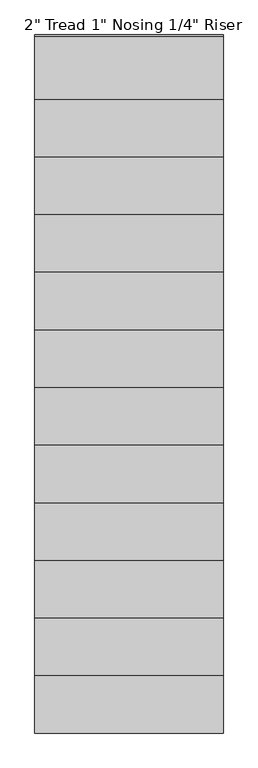
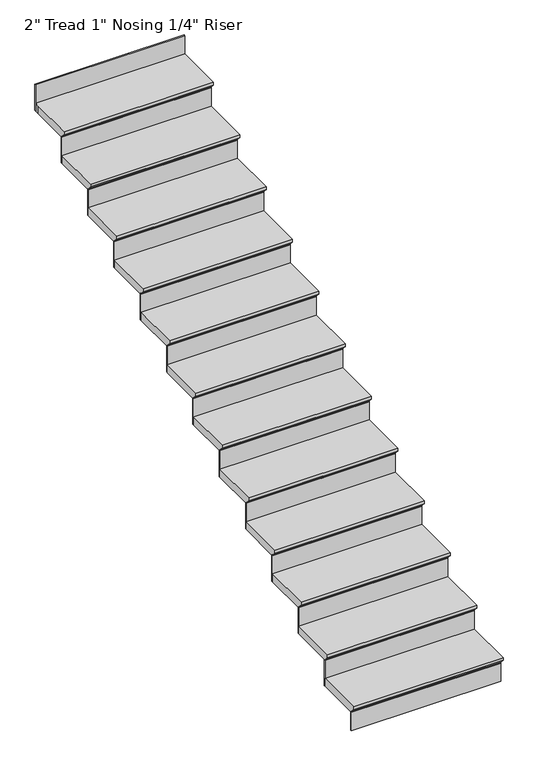
"""IFC4 building model written with IfcOpenShell, lengths in millimetres: stair flight geometry."""

from ifc_helpers import new_model, si_unit, origin, place, context, project, spatial, faceted_brep, source, transform, mapped, element, save


def stair_flight_f72f160c(model_context):
    return source(origin(), model_context, "Body", "Brep", [
        faceted_brep([(-2703.0415084, 19841.9216096, 43672.9005799), (-2703.0415084, 19841.9216096, 43691.9505799), (-3617.4415084, 19841.9216096, 43691.9505799), (-3617.4415084, 19841.9216096, 43672.9005799), (-2703.0415084, 19867.3216096, 43647.5005799), (-3617.4415084, 19867.3216096, 43647.5005799), (-2703.0415084, 20146.7216096, 43691.9505799), (-3617.4415084, 20146.7216096, 43691.9505799), (-3617.4415084, 19867.3216096, 43641.1505799), (-3617.4415084, 20146.7216096, 43641.1505799), (-2703.0415084, 20146.7216096, 43641.1505799), (-2703.0415084, 19867.3216096, 43641.1505799)], [[[0, 1, 2, 3]], [[4, 0, 3, 5]], [[2, 1, 6, 7]], [[8, 9, 10, 11]], [[2, 7, 9, 8, 5, 3]], [[8, 11, 4, 5]], [[6, 1, 0, 4, 11, 10]], [[7, 6, 10, 9]]]),
        faceted_brep([(-2703.0415084, 19867.3216096, 43641.1505799), (-2703.0415084, 19867.3216096, 43522.6172466), (-2703.0415084, 19873.6716096, 43522.6172466), (-2703.0415084, 19873.6716096, 43641.1505799), (-3617.4415084, 19867.3216096, 43641.1505799), (-3617.4415084, 19873.6716096, 43641.1505799), (-3617.4415084, 19873.6716096, 43522.6172466), (-3617.4415084, 19867.3216096, 43522.6172466)], [[[0, 1, 2, 3]], [[4, 5, 6, 7]], [[1, 0, 4, 7]], [[2, 1, 7, 6]], [[3, 2, 6, 5]], [[0, 3, 5, 4]]]),
        faceted_brep([(-2703.0415084, 20146.7216096, 43810.4839133), (-2703.0415084, 20146.7216096, 43641.1505799), (-2703.0415084, 20153.0716096, 43641.1505799), (-2703.0415084, 20153.0716096, 43810.4839133), (-3617.4415084, 20146.7216096, 43810.4839133), (-3617.4415084, 20153.0716096, 43810.4839133), (-3617.4415084, 20153.0716096, 43641.1505799), (-3617.4415084, 20146.7216096, 43641.1505799)], [[[0, 1, 2, 3]], [[4, 5, 6, 7]], [[1, 0, 4, 7]], [[2, 1, 7, 6]], [[3, 2, 6, 5]], [[0, 3, 5, 4]]]),
        faceted_brep([(-3617.4415084, 20121.3216096, 43861.2839133), (-2703.0415084, 20121.3216096, 43861.2839133), (-2703.0415084, 20426.1216096, 43861.2839133), (-3617.4415084, 20426.1216096, 43861.2839133), (-3617.4415084, 20146.7216096, 43810.4839133), (-3617.4415084, 20426.1216096, 43810.4839133), (-2703.0415084, 20426.1216096, 43810.4839133), (-2703.0415084, 20146.7216096, 43810.4839133), (-3617.4415084, 20146.7216096, 43816.8339133), (-3617.4415084, 20121.3216096, 43842.2339133), (-2703.0415084, 20146.7216096, 43816.8339133), (-2703.0415084, 20121.3216096, 43842.2339133)], [[[0, 1, 2, 3]], [[4, 5, 6, 7]], [[0, 3, 5, 4, 8, 9]], [[4, 7, 10, 8]], [[2, 1, 11, 10, 7, 6]], [[3, 2, 6, 5]], [[11, 1, 0, 9]], [[10, 11, 9, 8]]]),
        faceted_brep([(-2703.0415084, 20426.1216096, 43979.8172466), (-2703.0415084, 20426.1216096, 43810.4839133), (-2703.0415084, 20432.4716096, 43810.4839133), (-2703.0415084, 20432.4716096, 43979.8172466), (-3617.4415084, 20426.1216096, 43979.8172466), (-3617.4415084, 20432.4716096, 43979.8172466), (-3617.4415084, 20432.4716096, 43810.4839133), (-3617.4415084, 20426.1216096, 43810.4839133)], [[[0, 1, 2, 3]], [[4, 5, 6, 7]], [[1, 0, 4, 7]], [[2, 1, 7, 6]], [[3, 2, 6, 5]], [[0, 3, 5, 4]]]),
        faceted_brep([(-3617.4415084, 20400.7216096, 44030.6172466), (-2703.0415084, 20400.7216096, 44030.6172466), (-2703.0415084, 20705.5216096, 44030.6172466), (-3617.4415084, 20705.5216096, 44030.6172466), (-3617.4415084, 20426.1216096, 43979.8172466), (-3617.4415084, 20705.5216096, 43979.8172466), (-2703.0415084, 20705.5216096, 43979.8172466), (-2703.0415084, 20426.1216096, 43979.8172466), (-3617.4415084, 20426.1216096, 43986.1672466), (-3617.4415084, 20400.7216096, 44011.5672466), (-2703.0415084, 20426.1216096, 43986.1672466), (-2703.0415084, 20400.7216096, 44011.5672466)], [[[0, 1, 2, 3]], [[4, 5, 6, 7]], [[0, 3, 5, 4, 8, 9]], [[4, 7, 10, 8]], [[2, 1, 11, 10, 7, 6]], [[3, 2, 6, 5]], [[11, 1, 0, 9]], [[10, 11, 9, 8]]]),
        faceted_brep([(-2703.0415084, 20705.5216096, 44149.1505799), (-2703.0415084, 20705.5216096, 43979.8172466), (-2703.0415084, 20711.8716096, 43979.8172466), (-2703.0415084, 20711.8716096, 44149.1505799), (-3617.4415084, 20705.5216096, 44149.1505799), (-3617.4415084, 20711.8716096, 44149.1505799), (-3617.4415084, 20711.8716096, 43979.8172466), (-3617.4415084, 20705.5216096, 43979.8172466)], [[[0, 1, 2, 3]], [[4, 5, 6, 7]], [[1, 0, 4, 7]], [[2, 1, 7, 6]], [[3, 2, 6, 5]], [[0, 3, 5, 4]]]),
        faceted_brep([(-3617.4415084, 20680.1216096, 44199.9505799), (-2703.0415084, 20680.1216096, 44199.9505799), (-2703.0415084, 20984.9216096, 44199.9505799), (-3617.4415084, 20984.9216096, 44199.9505799), (-3617.4415084, 20705.5216096, 44149.1505799), (-3617.4415084, 20984.9216096, 44149.1505799), (-2703.0415084, 20984.9216096, 44149.1505799), (-2703.0415084, 20705.5216096, 44149.1505799), (-3617.4415084, 20705.5216096, 44155.5005799), (-3617.4415084, 20680.1216096, 44180.9005799), (-2703.0415084, 20705.5216096, 44155.5005799), (-2703.0415084, 20680.1216096, 44180.9005799)], [[[0, 1, 2, 3]], [[4, 5, 6, 7]], [[0, 3, 5, 4, 8, 9]], [[4, 7, 10, 8]], [[2, 1, 11, 10, 7, 6]], [[3, 2, 6, 5]], [[11, 1, 0, 9]], [[10, 11, 9, 8]]]),
        faceted_brep([(-2703.0415084, 20984.9216096, 44318.4839133), (-2703.0415084, 20984.9216096, 44149.1505799), (-2703.0415084, 20991.2716096, 44149.1505799), (-2703.0415084, 20991.2716096, 44318.4839133), (-3617.4415084, 20984.9216096, 44318.4839133), (-3617.4415084, 20991.2716096, 44318.4839133), (-3617.4415084, 20991.2716096, 44149.1505799), (-3617.4415084, 20984.9216096, 44149.1505799)], [[[0, 1, 2, 3]], [[4, 5, 6, 7]], [[1, 0, 4, 7]], [[2, 1, 7, 6]], [[3, 2, 6, 5]], [[0, 3, 5, 4]]]),
        faceted_brep([(-3617.4415084, 20959.5216096, 44369.2839133), (-2703.0415084, 20959.5216096, 44369.2839133), (-2703.0415084, 21264.3216096, 44369.2839133), (-3617.4415084, 21264.3216096, 44369.2839133), (-3617.4415084, 20984.9216096, 44318.4839133), (-3617.4415084, 21264.3216096, 44318.4839133), (-2703.0415084, 21264.3216096, 44318.4839133), (-2703.0415084, 20984.9216096, 44318.4839133), (-3617.4415084, 20984.9216096, 44324.8339133), (-3617.4415084, 20959.5216096, 44350.2339133), (-2703.0415084, 20984.9216096, 44324.8339133), (-2703.0415084, 20959.5216096, 44350.2339133)], [[[0, 1, 2, 3]], [[4, 5, 6, 7]], [[0, 3, 5, 4, 8, 9]], [[4, 7, 10, 8]], [[2, 1, 11, 10, 7, 6]], [[3, 2, 6, 5]], [[11, 1, 0, 9]], [[10, 11, 9, 8]]]),
        faceted_brep([(-2703.0415084, 21264.3216096, 44487.8172466), (-2703.0415084, 21264.3216096, 44318.4839133), (-2703.0415084, 21270.6716096, 44318.4839133), (-2703.0415084, 21270.6716096, 44487.8172466), (-3617.4415084, 21264.3216096, 44487.8172466), (-3617.4415084, 21270.6716096, 44487.8172466), (-3617.4415084, 21270.6716096, 44318.4839133), (-3617.4415084, 21264.3216096, 44318.4839133)], [[[0, 1, 2, 3]], [[4, 5, 6, 7]], [[1, 0, 4, 7]], [[2, 1, 7, 6]], [[3, 2, 6, 5]], [[0, 3, 5, 4]]]),
        faceted_brep([(-3617.4415084, 21238.9216096, 44538.6172466), (-2703.0415084, 21238.9216096, 44538.6172466), (-2703.0415084, 21543.7216096, 44538.6172466), (-3617.4415084, 21543.7216096, 44538.6172466), (-3617.4415084, 21264.3216096, 44487.8172466), (-3617.4415084, 21543.7216096, 44487.8172466), (-2703.0415084, 21543.7216096, 44487.8172466), (-2703.0415084, 21264.3216096, 44487.8172466), (-3617.4415084, 21264.3216096, 44494.1672466), (-3617.4415084, 21238.9216096, 44519.5672466), (-2703.0415084, 21264.3216096, 44494.1672466), (-2703.0415084, 21238.9216096, 44519.5672466)], [[[0, 1, 2, 3]], [[4, 5, 6, 7]], [[0, 3, 5, 4, 8, 9]], [[4, 7, 10, 8]], [[2, 1, 11, 10, 7, 6]], [[3, 2, 6, 5]], [[11, 1, 0, 9]], [[10, 11, 9, 8]]]),
        faceted_brep([(-2703.0415084, 21543.7216096, 44657.1505799), (-2703.0415084, 21543.7216096, 44487.8172466), (-2703.0415084, 21550.0716096, 44487.8172466), (-2703.0415084, 21550.0716096, 44657.1505799), (-3617.4415084, 21543.7216096, 44657.1505799), (-3617.4415084, 21550.0716096, 44657.1505799), (-3617.4415084, 21550.0716096, 44487.8172466), (-3617.4415084, 21543.7216096, 44487.8172466)], [[[0, 1, 2, 3]], [[4, 5, 6, 7]], [[1, 0, 4, 7]], [[2, 1, 7, 6]], [[3, 2, 6, 5]], [[0, 3, 5, 4]]]),
        faceted_brep([(-3617.4415084, 21518.3216096, 44707.9505799), (-2703.0415084, 21518.3216096, 44707.9505799), (-2703.0415084, 21823.1216096, 44707.9505799), (-3617.4415084, 21823.1216096, 44707.9505799), (-3617.4415084, 21543.7216096, 44657.1505799), (-3617.4415084, 21823.1216096, 44657.1505799), (-2703.0415084, 21823.1216096, 44657.1505799), (-2703.0415084, 21543.7216096, 44657.1505799), (-3617.4415084, 21543.7216096, 44663.5005799), (-3617.4415084, 21518.3216096, 44688.9005799), (-2703.0415084, 21543.7216096, 44663.5005799), (-2703.0415084, 21518.3216096, 44688.9005799)], [[[0, 1, 2, 3]], [[4, 5, 6, 7]], [[0, 3, 5, 4, 8, 9]], [[4, 7, 10, 8]], [[2, 1, 11, 10, 7, 6]], [[3, 2, 6, 5]], [[11, 1, 0, 9]], [[10, 11, 9, 8]]]),
        faceted_brep([(-2703.0415084, 21823.1216096, 44826.4839133), (-2703.0415084, 21823.1216096, 44657.1505799), (-2703.0415084, 21829.4716096, 44657.1505799), (-2703.0415084, 21829.4716096, 44826.4839133), (-3617.4415084, 21823.1216096, 44826.4839133), (-3617.4415084, 21829.4716096, 44826.4839133), (-3617.4415084, 21829.4716096, 44657.1505799), (-3617.4415084, 21823.1216096, 44657.1505799)], [[[0, 1, 2, 3]], [[4, 5, 6, 7]], [[1, 0, 4, 7]], [[2, 1, 7, 6]], [[3, 2, 6, 5]], [[0, 3, 5, 4]]]),
        faceted_brep([(-3617.4415084, 21797.7216096, 44877.2839133), (-2703.0415084, 21797.7216096, 44877.2839133), (-2703.0415084, 22102.5216096, 44877.2839133), (-3617.4415084, 22102.5216096, 44877.2839133), (-3617.4415084, 21823.1216096, 44826.4839133), (-3617.4415084, 22102.5216096, 44826.4839133), (-2703.0415084, 22102.5216096, 44826.4839133), (-2703.0415084, 21823.1216096, 44826.4839133), (-3617.4415084, 21823.1216096, 44832.8339133), (-3617.4415084, 21797.7216096, 44858.2339133), (-2703.0415084, 21823.1216096, 44832.8339133), (-2703.0415084, 21797.7216096, 44858.2339133)], [[[0, 1, 2, 3]], [[4, 5, 6, 7]], [[0, 3, 5, 4, 8, 9]], [[4, 7, 10, 8]], [[2, 1, 11, 10, 7, 6]], [[3, 2, 6, 5]], [[11, 1, 0, 9]], [[10, 11, 9, 8]]]),
        faceted_brep([(-2703.0415084, 22102.5216096, 44995.8172466), (-2703.0415084, 22102.5216096, 44826.4839133), (-2703.0415084, 22108.8716096, 44826.4839133), (-2703.0415084, 22108.8716096, 44995.8172466), (-3617.4415084, 22102.5216096, 44995.8172466), (-3617.4415084, 22108.8716096, 44995.8172466), (-3617.4415084, 22108.8716096, 44826.4839133), (-3617.4415084, 22102.5216096, 44826.4839133)], [[[0, 1, 2, 3]], [[4, 5, 6, 7]], [[1, 0, 4, 7]], [[2, 1, 7, 6]], [[3, 2, 6, 5]], [[0, 3, 5, 4]]]),
        faceted_brep([(-3617.4415084, 22077.1216096, 45046.6172466), (-2703.0415084, 22077.1216096, 45046.6172466), (-2703.0415084, 22381.9216096, 45046.6172466), (-3617.4415084, 22381.9216096, 45046.6172466), (-3617.4415084, 22102.5216096, 44995.8172466), (-3617.4415084, 22381.9216096, 44995.8172466), (-2703.0415084, 22381.9216096, 44995.8172466), (-2703.0415084, 22102.5216096, 44995.8172466), (-3617.4415084, 22102.5216096, 45002.1672466), (-3617.4415084, 22077.1216096, 45027.5672466), (-2703.0415084, 22102.5216096, 45002.1672466), (-2703.0415084, 22077.1216096, 45027.5672466)], [[[0, 1, 2, 3]], [[4, 5, 6, 7]], [[0, 3, 5, 4, 8, 9]], [[4, 7, 10, 8]], [[2, 1, 11, 10, 7, 6]], [[3, 2, 6, 5]], [[11, 1, 0, 9]], [[10, 11, 9, 8]]]),
        faceted_brep([(-2703.0415084, 22381.9216096, 45165.1505799), (-2703.0415084, 22381.9216096, 44995.8172466), (-2703.0415084, 22388.2716096, 44995.8172466), (-2703.0415084, 22388.2716096, 45165.1505799), (-3617.4415084, 22381.9216096, 45165.1505799), (-3617.4415084, 22388.2716096, 45165.1505799), (-3617.4415084, 22388.2716096, 44995.8172466), (-3617.4415084, 22381.9216096, 44995.8172466)], [[[0, 1, 2, 3]], [[4, 5, 6, 7]], [[1, 0, 4, 7]], [[2, 1, 7, 6]], [[3, 2, 6, 5]], [[0, 3, 5, 4]]]),
        faceted_brep([(-3617.4415084, 22356.5216096, 45215.9505799), (-2703.0415084, 22356.5216096, 45215.9505799), (-2703.0415084, 22661.3216096, 45215.9505799), (-3617.4415084, 22661.3216096, 45215.9505799), (-3617.4415084, 22381.9216096, 45165.1505799), (-3617.4415084, 22661.3216096, 45165.1505799), (-2703.0415084, 22661.3216096, 45165.1505799), (-2703.0415084, 22381.9216096, 45165.1505799), (-3617.4415084, 22381.9216096, 45171.5005799), (-3617.4415084, 22356.5216096, 45196.9005799), (-2703.0415084, 22381.9216096, 45171.5005799), (-2703.0415084, 22356.5216096, 45196.9005799)], [[[0, 1, 2, 3]], [[4, 5, 6, 7]], [[0, 3, 5, 4, 8, 9]], [[4, 7, 10, 8]], [[2, 1, 11, 10, 7, 6]], [[3, 2, 6, 5]], [[11, 1, 0, 9]], [[10, 11, 9, 8]]]),
        faceted_brep([(-2703.0415084, 22661.3216096, 45334.4839133), (-2703.0415084, 22661.3216096, 45165.1505799), (-2703.0415084, 22667.6716096, 45165.1505799), (-2703.0415084, 22667.6716096, 45334.4839133), (-3617.4415084, 22661.3216096, 45334.4839133), (-3617.4415084, 22667.6716096, 45334.4839133), (-3617.4415084, 22667.6716096, 45165.1505799), (-3617.4415084, 22661.3216096, 45165.1505799)], [[[0, 1, 2, 3]], [[4, 5, 6, 7]], [[1, 0, 4, 7]], [[2, 1, 7, 6]], [[3, 2, 6, 5]], [[0, 3, 5, 4]]]),
        faceted_brep([(-3617.4415084, 22635.9216096, 45385.2839133), (-2703.0415084, 22635.9216096, 45385.2839133), (-2703.0415084, 22940.7216096, 45385.2839133), (-3617.4415084, 22940.7216096, 45385.2839133), (-3617.4415084, 22661.3216096, 45334.4839133), (-3617.4415084, 22940.7216096, 45334.4839133), (-2703.0415084, 22940.7216096, 45334.4839133), (-2703.0415084, 22661.3216096, 45334.4839133), (-3617.4415084, 22661.3216096, 45340.8339133), (-3617.4415084, 22635.9216096, 45366.2339133), (-2703.0415084, 22661.3216096, 45340.8339133), (-2703.0415084, 22635.9216096, 45366.2339133)], [[[0, 1, 2, 3]], [[4, 5, 6, 7]], [[0, 3, 5, 4, 8, 9]], [[4, 7, 10, 8]], [[2, 1, 11, 10, 7, 6]], [[3, 2, 6, 5]], [[11, 1, 0, 9]], [[10, 11, 9, 8]]]),
        faceted_brep([(-2703.0415084, 23220.1216096, 45673.1505799), (-2703.0415084, 23220.1216096, 45503.8172466), (-2703.0415084, 23226.4716096, 45503.8172466), (-2703.0415084, 23226.4716096, 45673.1505799), (-3617.4415084, 23220.1216096, 45673.1505799), (-3617.4415084, 23226.4716096, 45673.1505799), (-3617.4415084, 23226.4716096, 45503.8172466), (-3617.4415084, 23220.1216096, 45503.8172466)], [[[0, 1, 2, 3]], [[4, 5, 6, 7]], [[1, 0, 4, 7]], [[2, 1, 7, 6]], [[3, 2, 6, 5]], [[0, 3, 5, 4]]]),
        faceted_brep([(-2703.0415084, 22940.7216096, 45503.8172466), (-2703.0415084, 22940.7216096, 45334.4839133), (-2703.0415084, 22947.0716096, 45334.4839133), (-2703.0415084, 22947.0716096, 45503.8172466), (-3617.4415084, 22940.7216096, 45503.8172466), (-3617.4415084, 22947.0716096, 45503.8172466), (-3617.4415084, 22947.0716096, 45334.4839133), (-3617.4415084, 22940.7216096, 45334.4839133)], [[[0, 1, 2, 3]], [[4, 5, 6, 7]], [[1, 0, 4, 7]], [[2, 1, 7, 6]], [[3, 2, 6, 5]], [[0, 3, 5, 4]]]),
        faceted_brep([(-3617.4415084, 23220.1216096, 45554.6172466), (-3617.4415084, 23194.7216096, 45554.6172466), (-3617.4415084, 22915.3216096, 45554.6172466), (-2703.0415084, 22915.3216096, 45554.6172466), (-2703.0415084, 23220.1216096, 45554.6172466), (-3617.4415084, 23194.7216096, 45503.8172466), (-3617.4415084, 23220.1216096, 45503.8172466), (-2703.0415084, 23220.1216096, 45503.8172466), (-2703.0415084, 22940.7216096, 45503.8172466), (-3617.4415084, 22940.7216096, 45503.8172466), (-3617.4415084, 22940.7216096, 45510.1672466), (-3617.4415084, 22915.3216096, 45535.5672466), (-2703.0415084, 22940.7216096, 45510.1672466), (-2703.0415084, 22915.3216096, 45535.5672466)], [[[0, 1, 2, 3, 4]], [[5, 6, 7, 8, 9]], [[1, 0, 6, 5]], [[2, 1, 5, 9, 10, 11]], [[9, 8, 12, 10]], [[4, 3, 13, 12, 8, 7]], [[0, 4, 7, 6]], [[13, 3, 2, 11]], [[12, 13, 11, 10]]]),
    ])


if __name__ == "__main__":
    model = new_model("IFC4")
    model_context = context("Model", 3, world=origin())
    ifc_project = project(units=[si_unit("LENGTHUNIT", "METRE", prefix="MILLI")], contexts=[model_context])
    site = spatial("IfcSite", under=ifc_project)
    building = spatial("IfcBuilding", under=site)
    placement = place(None, origin())
    stair_flight_shape = stair_flight_f72f160c(model_context)
    element("IfcStairFlight", 1, ObjectType="2\" Tread 1\" Nosing 1/4\" Riser", at=placement, inside=building, context=model_context, shape_type="MappedRepresentation", body=[
        mapped(stair_flight_shape, transform((0.0, 0.0, 0.0), x_axis=(1.0, 0.0, 0.0), y_axis=(0.0, 1.0, 0.0), z_axis=(0.0, 0.0, 1.0))),
    ])
    save(model, "model.ifc")
